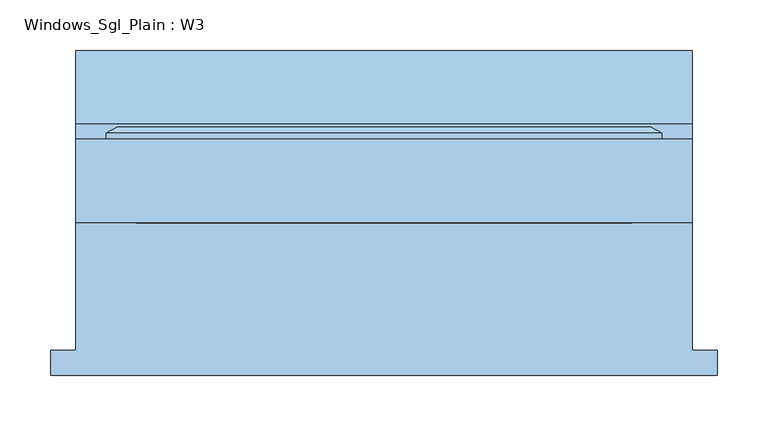
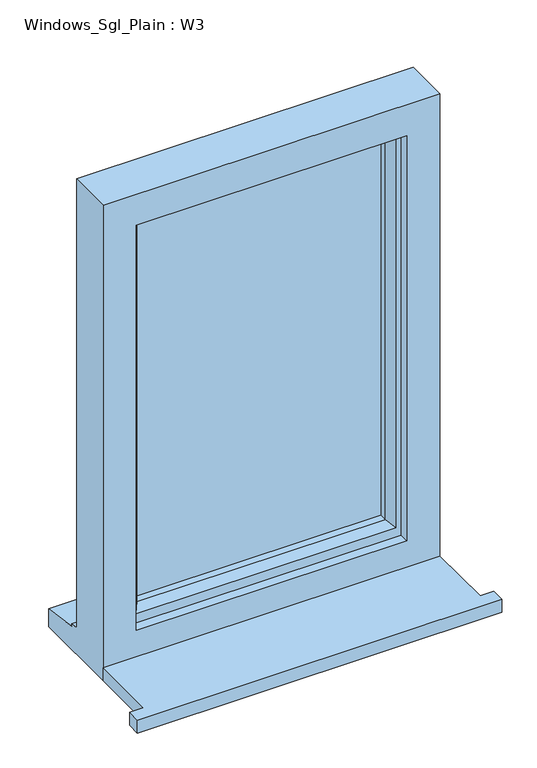
"""IFC4 building model written with IfcOpenShell, lengths in millimetres: window geometry, Windows_Sgl_Plain : W3."""

from ifc_helpers import new_model, si_unit, frame, origin, place, context, project, spatial, polyline, outline, extrude, faceted_brep, source, transform, mapped, element, save


def windows_sgl_plain_w3_3107c001(model_context):
    return source(origin(), model_context, "Body", "SolidModel", [
        extrude(outline(polyline([(-329.8, -146.0834322), (-329.8, -121.0834322), (-304.8, -121.0834322), (-304.8, 4.9965678), (304.8, 4.9965678), (304.8, -121.0834322), (329.8, -121.0834322), (329.8, -146.0834322), (-329.8, -146.0834322)])), frame((0.0, 0.0, 1200.0), z_axis=(0.0, 0.0, 1.0), x_axis=(1.0, 0.0, 0.0)), (0.0, 0.0, 1.0), 25.0),
        faceted_brep([(-304.8, 4.9965678, 1200.0), (304.8, 4.9965678, 1200.0), (304.8, 4.9965678, 2110.0), (-304.8, 4.9965678, 2110.0), (-244.8, 4.9965678, 2050.0), (244.8, 4.9965678, 2050.0), (244.8, 4.9965678, 1275.0), (-244.8, 4.9965678, 1275.0), (-304.8, 87.9965678, 2110.0), (-304.8, 87.9965678, 1251.0), (-304.8, 102.9965678, 1249.68767), (-304.8, 102.9965678, 1244.7449676), (-304.8, 175.4965678, 1233.8088847), (-304.8, 175.4965678, 1200.0), (304.8, 87.9965678, 2110.0), (304.8, 87.9965678, 1251.0), (-264.8, 87.9965678, 2070.0), (-264.8, 87.9965678, 1263.0), (264.8, 87.9965678, 1263.0), (264.8, 87.9965678, 2070.0), (-264.8, 22.9965678, 2070.0), (-264.8, 22.9965678, 1263.0), (264.8, 22.9965678, 2070.0), (264.8, 22.9965678, 1263.0), (-244.8, 22.9965678, 2050.0), (-244.8, 22.9965678, 1275.0), (244.8, 22.9965678, 1275.0), (244.8, 22.9965678, 2050.0), (304.8, 175.4965678, 1200.0), (304.8, 175.4965678, 1233.8088847), (304.8, 102.9965678, 1244.7449676), (304.8, 102.9965678, 1249.68767)], [[[0, 1, 2, 3], [4, 5, 6, 7]], [[0, 3, 8, 9, 10, 11, 12, 13]], [[9, 8, 14, 15], [16, 17, 18, 19]], [[17, 16, 20, 21]], [[20, 22, 23, 21], [24, 25, 26, 27]], [[24, 4, 7, 25]], [[3, 2, 14, 8]], [[16, 19, 22, 20]], [[5, 4, 24, 27]], [[15, 14, 2, 1, 28, 29, 30, 31]], [[19, 18, 23, 22]], [[5, 27, 26, 6]], [[28, 1, 0, 13]], [[29, 28, 13, 12]], [[30, 29, 12, 11]], [[31, 30, 11, 10]], [[15, 31, 10, 9]], [[21, 23, 18, 17]], [[7, 6, 26, 25]]]),
        extrude(outline(polyline([(234.8, 51.9965678), (-234.8, 51.9965678), (-234.8, 75.9965678), (234.8, 75.9965678), (234.8, 51.9965678)])), frame((0.0, 0.0, 1293.0), z_axis=(0.0, 0.0, 1.0), x_axis=(1.0, 0.0, 0.0)), (0.0, 0.0, 1.0), 747.0),
        faceted_brep([(-274.8, 87.9965678, 2080.0), (-274.8, 93.7700705, 2080.0), (-274.8, 93.7700705, 1253.0), (-274.8, 87.9965678, 1253.0), (-264.8, 22.9965678, 2070.0), (-264.8, 87.9965678, 2070.0), (-264.8, 87.9965678, 1263.0), (-264.8, 22.9965678, 1263.0), (-224.8, 37.4894677, 2030.0), (-234.9480377, 22.9965678, 2040.1480377), (-234.9480377, 22.9965678, 1292.8519623), (-224.8, 37.4894677, 1303.0), (-224.8, 51.9965678, 2030.0), (-224.8, 51.9965678, 1303.0), (-234.8, 75.9965678, 2040.0), (-234.8, 51.9965678, 2040.0), (-234.8, 51.9965678, 1293.0), (-234.8, 75.9965678, 1293.0), (-224.8, 93.7700705, 2030.0), (-224.8, 75.9965678, 2030.0), (-224.8, 75.9965678, 1303.0), (-224.8, 93.7700705, 1303.0), (-242.2457548, 99.5435732, 2047.4457548), (-242.2457548, 99.5435732, 1285.5542452), (-264.0153903, 99.5435732, 2069.2153903), (-264.0153903, 99.5435732, 1263.7846097), (274.8, 93.7700705, 1253.0), (274.8, 87.9965678, 1253.0), (264.8, 87.9965678, 1263.0), (264.8, 22.9965678, 1263.0), (234.9480377, 22.9965678, 1292.8519623), (224.8, 37.4894677, 1303.0), (224.8, 51.9965678, 1303.0), (234.8, 51.9965678, 1293.0), (234.8, 75.9965678, 1293.0), (224.8, 75.9965678, 1303.0), (224.8, 93.7700705, 1303.0), (242.2457548, 99.5435732, 1285.5542452), (264.0153903, 99.5435732, 1263.7846097), (274.8, 93.7700705, 2080.0), (274.8, 87.9965678, 2080.0), (264.8, 87.9965678, 2070.0), (264.8, 22.9965678, 2070.0), (234.9480377, 22.9965678, 2040.1480377), (224.8, 37.4894677, 2030.0), (224.8, 51.9965678, 2030.0), (234.8, 51.9965678, 2040.0), (234.8, 75.9965678, 2040.0), (224.8, 75.9965678, 2030.0), (224.8, 93.7700705, 2030.0), (242.2457548, 99.5435732, 2047.4457548), (264.0153903, 99.5435732, 2069.2153903)], [[[0, 1, 2, 3]], [[4, 5, 6, 7]], [[8, 9, 10, 11]], [[12, 8, 11, 13]], [[14, 15, 16, 17]], [[18, 19, 20, 21]], [[22, 18, 21, 23]], [[1, 24, 25, 2]], [[3, 2, 26, 27]], [[7, 6, 28, 29]], [[11, 10, 30, 31]], [[13, 11, 31, 32]], [[17, 16, 33, 34]], [[21, 20, 35, 36]], [[23, 21, 36, 37]], [[2, 25, 38, 26]], [[27, 26, 39, 40]], [[29, 28, 41, 42]], [[31, 30, 43, 44]], [[32, 31, 44, 45]], [[34, 33, 46, 47]], [[36, 35, 48, 49]], [[37, 36, 49, 50]], [[26, 38, 51, 39]], [[40, 39, 1, 0]], [[3, 27, 40, 0], [5, 41, 28, 6]], [[42, 41, 5, 4]], [[7, 29, 42, 4], [9, 43, 30, 10]], [[44, 43, 9, 8]], [[45, 44, 8, 12]], [[15, 46, 33, 16], [13, 32, 45, 12]], [[47, 46, 15, 14]], [[17, 34, 47, 14], [19, 48, 35, 20]], [[49, 48, 19, 18]], [[50, 49, 18, 22]], [[24, 51, 38, 25], [23, 37, 50, 22]], [[39, 51, 24, 1]]]),
    ])


if __name__ == "__main__":
    model = new_model("IFC4")
    model_context = context("Model", 3, world=origin())
    ifc_project = project(units=[si_unit("LENGTHUNIT", "METRE", prefix="MILLI")], contexts=[model_context])
    site = spatial("IfcSite", under=ifc_project)
    building = spatial("IfcBuilding", under=site)
    placement = place(None, origin())
    windows_sgl_plain_w3_shape = windows_sgl_plain_w3_3107c001(model_context)
    element("IfcWindow", 1, ObjectType="Windows_Sgl_Plain : W3", at=placement, inside=building, context=model_context, shape_type="MappedRepresentation", body=[
        mapped(windows_sgl_plain_w3_shape, transform((0.0, 0.0, 0.0), x_axis=(1.0, 0.0, 0.0), y_axis=(0.0, 1.0, 0.0), z_axis=(0.0, 0.0, 1.0))),
    ])
    save(model, "model.ifc")

# Revit data of these elements
# Type "Windows_Sgl_Plain : W3"
#   Type Mark = "58"
#   Operation = "SinglePanel"
#   Construction Type Id = "SGL"
#   Manufacturer = "Revit"
#   Keynote = "L10"
#   Analytic Construction = "Large single-glazed windows"
#   Wrap Layers (Ext) from Ext = 102.5 mm
#   Wrap Layers (Int) from Ext = 177.5 mm
#   Window Board Projection = 25 mm
#   Window Board Extension = 25 mm
#   Visual Light Transmittance = 0.9
#   Solar Heat Gain Coefficient = 0.86
#   Rough Width = 609.6 mm
#   Rough Height = 910 mm
#   Height = 910 mm
#   Width = 609.6 mm
#   Heat Transfer Coefficient (U) = 5.5617 W/(m²·K)
#   Glazing Thickness = 24 mm
#   FrameOffset - External = 50 mm
#   Frame Depth = 65 mm
#   Default Head Height = 2110 mm
#   Cill Depth = 87.5 mm
#   Cavity Closer Width = 50 mm
#   Cavity Closer Offset from Ext = 102.5 mm
#   Cavity Closer Depth = 85 mm
#   Vis - Cavity Closers = yes
#   Define Thermal Properties by = 1
#   Material Trim = Window Frame
#   Material Glass = Glass
#   Material Frame = Window Frame
#   Wall Closure = (empty or 0)
# Element 1 (IfcWindow, "Windows_Sgl_Plain : W3")
#   Materials on its faces: "Window Frame", "Glass"
# Materials
#   "Window Frame": colour RGB 249 249 249, transparency 0, Keynote = "L10", Cost = 0
#   "Glass": class "Glass", colour RGB 0 128 192, transparency 0.9, Description = "Soda Lime Glass", Cost = 0
